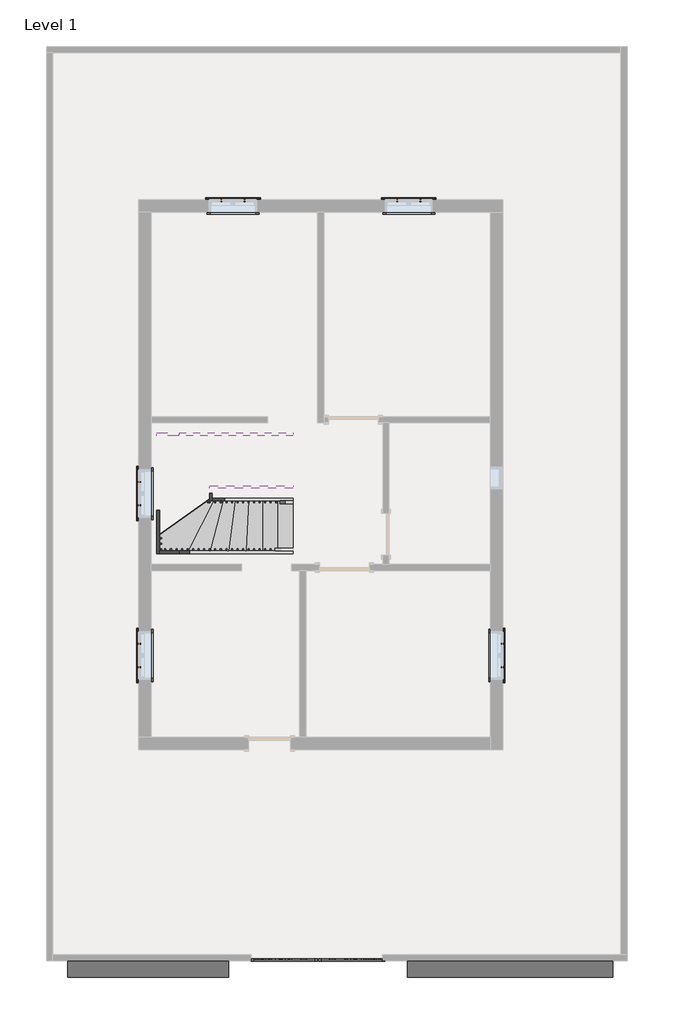
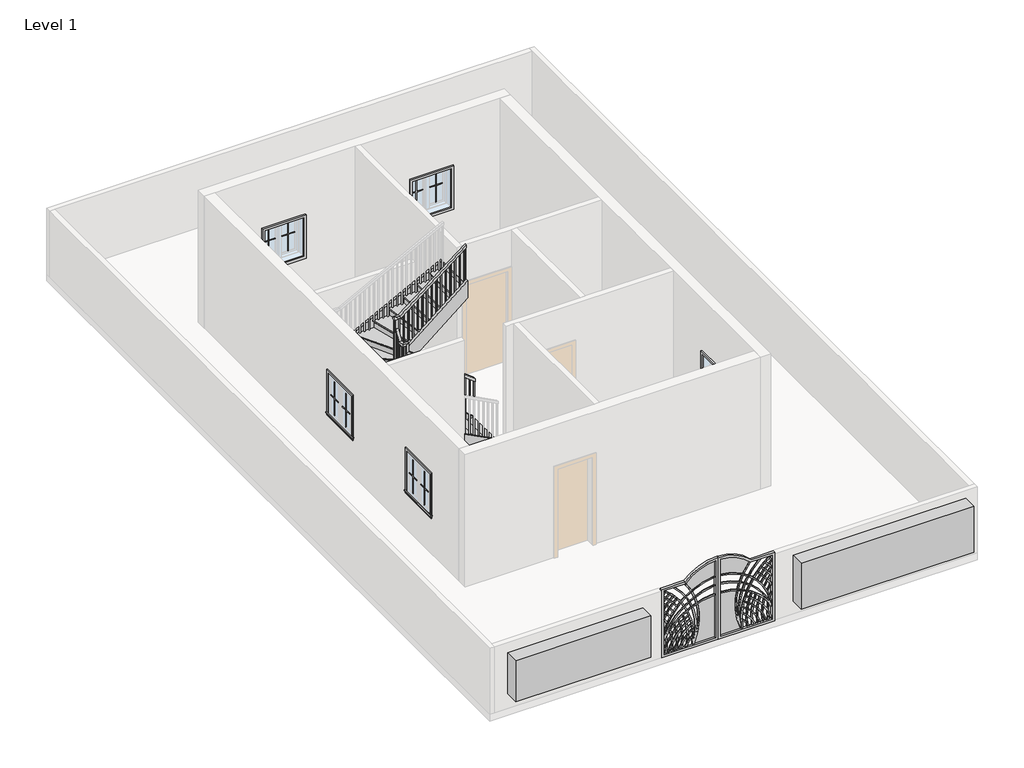
# One storey, part 2 of 2: 22 proxies, 8 members, 1 railing, 1 stair flight.
"""IFC4 building model written with IfcOpenShell, lengths in millimetres."""

from ifc_helpers import new_model, si_unit, frame, origin, place, context, project, spatial, polyline, outline, extrude, faceted_brep, transform, mapped, element, save
from components import generic_models_6bc30956, generic_models_1_generic_models_1_64d4bc32, muntin_pattern_2x2_muntin_pattern_2x2_b3fe6957, muntin_pattern_2x2_muntin_pattern_2x2_3e0ecaf2, trim_window_exterior_flat_with_sill_41619996, trim_window_interior_flat_picture_frame_51c85655, stair_flight_6f16d7d9

model = new_model("IFC4")

# Units and contexts
model_context = context("Model", 3, world=origin())
ifc_project = project(units=[si_unit("LENGTHUNIT", "METRE", prefix="MILLI")], contexts=[model_context])

# Site, building, storey
site = spatial("IfcSite", under=ifc_project)
building = spatial("IfcBuilding", under=site)
storey = spatial("IfcBuildingStorey", under=building, Name="Level 1", Elevation=0.0)

# Proxies
placement = place(None, origin())
generic_models_shape = generic_models_6bc30956(model_context)
element("IfcBuildingElementProxy", 1, Name="Generic Models", at=placement, inside=storey, context=model_context, shape_type="MappedRepresentation", body=[
    mapped(generic_models_shape, transform((-1329.9449167, -8721.9675636, 0.0), x_axis=(1.0, 0.0, 0.0), y_axis=(0.0, 1.0, 0.0), z_axis=(0.0, 0.0, 1.0))),
])
generic_models_1_generic_models_1_shape = generic_models_1_generic_models_1_64d4bc32(model_context)
element("IfcBuildingElementProxy", 2, Name="Generic Models 1 : Generic Models 1", ObjectType="Generic Models 1 : Generic Models 1", at=placement, inside=storey, context=model_context, shape_type="MappedRepresentation", body=[
    mapped(generic_models_1_generic_models_1_shape, transform((0.0, 0.0, 0.0), x_axis=(1.0, 0.0, 0.0), y_axis=(0.0, 1.0, 0.0), z_axis=(0.0, 0.0, 1.0))),
])
muntin_pattern_2x2_muntin_pattern_2x2_shape = muntin_pattern_2x2_muntin_pattern_2x2_b3fe6957(model_context)
element("IfcBuildingElementProxy", 3, Name="Muntin Pattern_2x2 : Muntin Pattern_2x2", ObjectType="Muntin Pattern_2x2 : Muntin Pattern_2x2", at=placement, inside=storey, context=model_context, shape_type="MappedRepresentation", body=[
    mapped(muntin_pattern_2x2_muntin_pattern_2x2_shape, transform((-3096.8324167, 5150.2179147, 984.25), x_axis=(1.0, 0.0, 0.0), y_axis=(0.0, 1.0, 0.0), z_axis=(0.0, 0.0, 1.0))),
])
element("IfcBuildingElementProxy", 4, Name="Muntin Pattern_2x2 : Muntin Pattern_2x2", ObjectType="Muntin Pattern_2x2 : Muntin Pattern_2x2", at=placement, inside=storey, context=model_context, shape_type="MappedRepresentation", body=[
    mapped(muntin_pattern_2x2_muntin_pattern_2x2_shape, transform((122.6175833, 5150.2179147, 984.25), x_axis=(1.0, 0.0, 0.0), y_axis=(0.0, 1.0, 0.0), z_axis=(0.0, 0.0, 1.0))),
])
element("IfcBuildingElementProxy", 5, Name="Muntin Pattern_2x2 : Muntin Pattern_2x2", ObjectType="Muntin Pattern_2x2 : Muntin Pattern_2x2", at=placement, inside=storey, context=model_context, shape_type="MappedRepresentation", body=[
    mapped(muntin_pattern_2x2_muntin_pattern_2x2_shape, transform((2051.4300833, -2960.3195853, 984.25), x_axis=(0.0, -1.0, 0.0), y_axis=(1.0, 0.0, 0.0), z_axis=(0.0, 0.0, 1.0))),
])
element("IfcBuildingElementProxy", 6, Name="Muntin Pattern_2x2 : Muntin Pattern_2x2", ObjectType="Muntin Pattern_2x2 : Muntin Pattern_2x2", at=placement, inside=storey, context=model_context, shape_type="MappedRepresentation", body=[
    mapped(muntin_pattern_2x2_muntin_pattern_2x2_shape, transform((-4597.0199167, -3388.9445853, 984.25), x_axis=(0.0, 1.0, 0.0), y_axis=(-1.0, 0.0, 0.0), z_axis=(0.0, 0.0, 1.0))),
])
element("IfcBuildingElementProxy", 7, Name="Muntin Pattern_2x2 : Muntin Pattern_2x2", ObjectType="Muntin Pattern_2x2 : Muntin Pattern_2x2", at=placement, inside=storey, context=model_context, shape_type="MappedRepresentation", body=[
    mapped(muntin_pattern_2x2_muntin_pattern_2x2_shape, transform((-4597.0199167, -426.6695853, 984.25), x_axis=(0.0, 1.0, 0.0), y_axis=(-1.0, 0.0, 0.0), z_axis=(0.0, 0.0, 1.0))),
])
muntin_pattern_2x2_muntin_pattern_2x2_2_shape = muntin_pattern_2x2_muntin_pattern_2x2_3e0ecaf2(model_context)
element("IfcBuildingElementProxy", 8, Name="Muntin Pattern_2x2 : Muntin Pattern_2x2", ObjectType="Muntin Pattern_2x2 : Muntin Pattern_2x2", at=placement, inside=storey, context=model_context, shape_type="MappedRepresentation", body=[
    mapped(muntin_pattern_2x2_muntin_pattern_2x2_2_shape, transform((-2668.2074167, 5150.2179147, 984.25), x_axis=(-1.0, 0.0, 0.0), y_axis=(0.0, -1.0, 0.0), z_axis=(0.0, 0.0, 1.0))),
])
element("IfcBuildingElementProxy", 9, Name="Muntin Pattern_2x2 : Muntin Pattern_2x2", ObjectType="Muntin Pattern_2x2 : Muntin Pattern_2x2", at=placement, inside=storey, context=model_context, shape_type="MappedRepresentation", body=[
    mapped(muntin_pattern_2x2_muntin_pattern_2x2_2_shape, transform((551.2425833, 5150.2179147, 984.25), x_axis=(-1.0, 0.0, 0.0), y_axis=(0.0, -1.0, 0.0), z_axis=(0.0, 0.0, 1.0))),
])
element("IfcBuildingElementProxy", 10, Name="Muntin Pattern_2x2 : Muntin Pattern_2x2", ObjectType="Muntin Pattern_2x2 : Muntin Pattern_2x2", at=placement, inside=storey, context=model_context, shape_type="MappedRepresentation", body=[
    mapped(muntin_pattern_2x2_muntin_pattern_2x2_2_shape, transform((2051.4300833, -3388.9445853, 984.25), x_axis=(0.0, 1.0, 0.0), y_axis=(-1.0, 0.0, 0.0), z_axis=(0.0, 0.0, 1.0))),
])
element("IfcBuildingElementProxy", 11, Name="Muntin Pattern_2x2 : Muntin Pattern_2x2", ObjectType="Muntin Pattern_2x2 : Muntin Pattern_2x2", at=placement, inside=storey, context=model_context, shape_type="MappedRepresentation", body=[
    mapped(muntin_pattern_2x2_muntin_pattern_2x2_2_shape, transform((-4597.0199167, -2960.3195853, 984.25), x_axis=(0.0, -1.0, 0.0), y_axis=(1.0, 0.0, 0.0), z_axis=(0.0, 0.0, 1.0))),
])
element("IfcBuildingElementProxy", 12, Name="Muntin Pattern_2x2 : Muntin Pattern_2x2", ObjectType="Muntin Pattern_2x2 : Muntin Pattern_2x2", at=placement, inside=storey, context=model_context, shape_type="MappedRepresentation", body=[
    mapped(muntin_pattern_2x2_muntin_pattern_2x2_2_shape, transform((-4597.0199167, 1.9554147, 984.25), x_axis=(0.0, -1.0, 0.0), y_axis=(1.0, 0.0, 0.0), z_axis=(0.0, 0.0, 1.0))),
])
trim_window_exterior_flat_with_sill_shape = trim_window_exterior_flat_with_sill_41619996(model_context)
element("IfcBuildingElementProxy", 13, Name="Trim-Window-Exterior-Flat : with Sill", ObjectType="Trim-Window-Exterior-Flat : with Sill", at=placement, inside=storey, context=model_context, shape_type="MappedRepresentation", body=[
    mapped(trim_window_exterior_flat_with_sill_shape, transform((-2882.5199167, 5159.7429147, 1828.8), x_axis=(-1.0, 0.0, 0.0), y_axis=(0.0, 0.0, 1.0), z_axis=(0.0, 1.0, 0.0))),
])
element("IfcBuildingElementProxy", 14, Name="Trim-Window-Exterior-Flat : with Sill", ObjectType="Trim-Window-Exterior-Flat : with Sill", at=placement, inside=storey, context=model_context, shape_type="MappedRepresentation", body=[
    mapped(trim_window_exterior_flat_with_sill_shape, transform((336.9300833, 5159.7429147, 1828.8), x_axis=(-1.0, 0.0, 0.0), y_axis=(0.0, 0.0, 1.0), z_axis=(0.0, 1.0, 0.0))),
])
element("IfcBuildingElementProxy", 15, Name="Trim-Window-Exterior-Flat : with Sill", ObjectType="Trim-Window-Exterior-Flat : with Sill", at=placement, inside=storey, context=model_context, shape_type="MappedRepresentation", body=[
    mapped(trim_window_exterior_flat_with_sill_shape, transform((2060.9550833, -3174.6320853, 1828.8), x_axis=(0.0, 1.0, 0.0), y_axis=(0.0, 0.0, 1.0), z_axis=(1.0, 0.0, 0.0))),
])
element("IfcBuildingElementProxy", 16, Name="Trim-Window-Exterior-Flat : with Sill", ObjectType="Trim-Window-Exterior-Flat : with Sill", at=placement, inside=storey, context=model_context, shape_type="MappedRepresentation", body=[
    mapped(trim_window_exterior_flat_with_sill_shape, transform((-4606.5449167, -3174.6320853, 1828.8), x_axis=(0.0, -1.0, 0.0), y_axis=(0.0, 0.0, 1.0), z_axis=(-1.0, 0.0, 0.0))),
])
element("IfcBuildingElementProxy", 17, Name="Trim-Window-Exterior-Flat : with Sill", ObjectType="Trim-Window-Exterior-Flat : with Sill", at=placement, inside=storey, context=model_context, shape_type="MappedRepresentation", body=[
    mapped(trim_window_exterior_flat_with_sill_shape, transform((-4606.5449167, -212.3570853, 1828.8), x_axis=(0.0, -1.0, 0.0), y_axis=(0.0, 0.0, 1.0), z_axis=(-1.0, 0.0, 0.0))),
])
trim_window_interior_flat_picture_frame_shape = trim_window_interior_flat_picture_frame_51c85655(model_context)
element("IfcBuildingElementProxy", 18, Name="Trim-Window-Interior-Flat : Picture Frame", ObjectType="Trim-Window-Interior-Flat : Picture Frame", at=placement, inside=storey, context=model_context, shape_type="MappedRepresentation", body=[
    mapped(trim_window_interior_flat_picture_frame_shape, transform((-2882.5199167, 4931.1429147, 1828.8), x_axis=(1.0, 0.0, 0.0), y_axis=(0.0, 0.0, 1.0), z_axis=(0.0, -1.0, 0.0))),
])
element("IfcBuildingElementProxy", 19, Name="Trim-Window-Interior-Flat : Picture Frame", ObjectType="Trim-Window-Interior-Flat : Picture Frame", at=placement, inside=storey, context=model_context, shape_type="MappedRepresentation", body=[
    mapped(trim_window_interior_flat_picture_frame_shape, transform((336.9300833, 4931.1429147, 1828.8), x_axis=(1.0, 0.0, 0.0), y_axis=(0.0, 0.0, 1.0), z_axis=(0.0, -1.0, 0.0))),
])
element("IfcBuildingElementProxy", 20, Name="Trim-Window-Interior-Flat : Picture Frame", ObjectType="Trim-Window-Interior-Flat : Picture Frame", at=placement, inside=storey, context=model_context, shape_type="MappedRepresentation", body=[
    mapped(trim_window_interior_flat_picture_frame_shape, transform((1832.3550833, -3174.6320853, 1828.8), x_axis=(0.0, -1.0, 0.0), y_axis=(0.0, 0.0, 1.0), z_axis=(-1.0, 0.0, 0.0))),
])
element("IfcBuildingElementProxy", 21, Name="Trim-Window-Interior-Flat : Picture Frame", ObjectType="Trim-Window-Interior-Flat : Picture Frame", at=placement, inside=storey, context=model_context, shape_type="MappedRepresentation", body=[
    mapped(trim_window_interior_flat_picture_frame_shape, transform((-4377.9449167, -3174.6320853, 1828.8), x_axis=(0.0, 1.0, 0.0), y_axis=(0.0, 0.0, 1.0), z_axis=(1.0, 0.0, 0.0))),
])
element("IfcBuildingElementProxy", 22, Name="Trim-Window-Interior-Flat : Picture Frame", ObjectType="Trim-Window-Interior-Flat : Picture Frame", at=placement, inside=storey, context=model_context, shape_type="MappedRepresentation", body=[
    mapped(trim_window_interior_flat_picture_frame_shape, transform((-4377.9449167, -212.3570853, 1828.8), x_axis=(0.0, 1.0, 0.0), y_axis=(0.0, 0.0, 1.0), z_axis=(1.0, 0.0, 0.0))),
])

# Members
element("IfcMember", 23, ObjectType="Stringer - 2\" Width", at=placement, inside=storey, context=model_context, shape_type="SweptSolid", body=[
    extrude(outline(polyline([(0.0, -1783.4132248), (229.639954, -1783.4132248), (1305.3956453, -3870.8304165), (962.500629, -3870.8304165), (0.0, -2003.1755424), (0.0, -1783.4132248)])), frame((0.0, -1310.9070853, 0.0), z_axis=(0.0, 1.0, 0.0), x_axis=(0.0, 0.0, 1.0)), (0.0, 0.0, 1.0), 50.8),
])
element("IfcMember", 24, ObjectType="Stringer - 2\" Width", at=placement, inside=storey, context=model_context, shape_type="SweptSolid", body=[
    extrude(outline(polyline([(-3870.8304165, -1260.1070853), (-3870.8304165, -1310.9070853), (-4225.5449167, -1310.9070853), (-4225.5449167, -1260.1070853), (-3870.8304165, -1260.1070853)])), frame((0.0, 0.0, 962.500629), z_axis=(0.0, 0.0, 1.0), x_axis=(1.0, 0.0, 0.0)), (0.0, 0.0, 1.0), 342.8950162),
])
element("IfcMember", 25, ObjectType="Stringer - 2\" Width", at=placement, inside=storey, context=model_context, shape_type="SweptSolid", body=[
    extrude(outline(polyline([(-1310.9070853, 1000.5956453), (-1310.9070853, 1289.0952212), (811.1127974, 1969.9972697), (848.0929147, 1969.9972697), (848.0929147, 1638.9682298), (-1141.3846024, 1000.5956453), (-1310.9070853, 1000.5956453)])), frame((-4276.3449167, 0.0, 0.0), z_axis=(1.0, 0.0, 0.0), x_axis=(0.0, 1.0, 0.0)), (0.0, 0.0, 1.0), 50.8),
])
element("IfcMember", 26, ObjectType="Stringer - 2\" Width", at=placement, inside=storey, context=model_context, shape_type="SweptSolid", body=[
    extrude(outline(polyline([(-4276.3449167, 848.0929147), (-4276.3449167, 898.8929147), (-3870.8304165, 898.8929147), (-3870.8304165, 848.0929147), (-4276.3449167, 848.0929147)])), frame((0.0, 0.0, 1649.8904473), z_axis=(0.0, 0.0, 1.0), x_axis=(1.0, 0.0, 0.0)), (0.0, 0.0, 1.0), 320.1068224),
])
element("IfcMember", 27, ObjectType="Stringer - 2\" Width", at=placement, inside=storey, context=model_context, shape_type="SweptSolid", body=[
    extrude(outline(polyline([(1969.9972697, -3870.8304165), (1649.8904473, -3870.8304165), (2725.6461385, -1783.4132248), (3045.7529609, -1783.4132248), (1969.9972697, -3870.8304165)])), frame((0.0, 848.0929147, 0.0), z_axis=(0.0, 1.0, 0.0), x_axis=(0.0, 0.0, 1.0)), (0.0, 0.0, 1.0), 50.8),
])
element("IfcMember", 28, ObjectType="Stringer - 2\" Width", at=placement, inside=storey, context=model_context, shape_type="SweptSolid", body=[
    extrude(outline(polyline([(0.0, -1783.4132248), (176.1764461, -1783.4132248), (1380.418648, -3260.3449167), (987.1410923, -3260.3449167), (0.0, -2049.6748694), (0.0, -1783.4132248)])), frame((0.0, -345.7070853, 0.0), z_axis=(0.0, 1.0, 0.0), x_axis=(0.0, 0.0, 1.0)), (0.0, 0.0, 1.0), 50.8),
])
element("IfcMember", 29, ObjectType="Stringer - 2\" Width", at=placement, inside=storey, context=model_context, shape_type="SweptSolid", body=[
    extrude(outline(polyline([(-345.7070853, 1028.5617647), (-345.7070853, 1573.2682978), (-139.0699679, 1926.1409689), (-117.1070853, 1926.1409689), (-117.1070853, 1360.465107), (-311.464868, 1028.5617647), (-345.7070853, 1028.5617647)])), frame((-3311.1449167, 0.0, 0.0), z_axis=(1.0, 0.0, 0.0), x_axis=(0.0, 1.0, 0.0)), (0.0, 0.0, 1.0), 50.8),
])
element("IfcMember", 30, ObjectType="Stringer - 2\" Width", at=placement, inside=storey, context=model_context, shape_type="SweptSolid", body=[
    extrude(outline(polyline([(1926.1409689, -3311.1449167), (1532.8634131, -3311.1449167), (2778.5262875, -1783.4132248), (3171.8038432, -1783.4132248), (1926.1409689, -3311.1449167)])), frame((0.0, -117.1070853, 0.0), z_axis=(0.0, 1.0, 0.0), x_axis=(0.0, 0.0, 1.0)), (0.0, 0.0, 1.0), 50.8),
])

# Railing
element("IfcRailing", 31, ObjectType="Handrail - Rectangular", at=placement, inside=storey, context=model_context, shape_type="SolidModel", body=[
    faceted_brep([(-1783.4132248, -396.5070853, 1083.7333333), (-1783.4132248, -396.5070853, 1019.4000346), (-1783.4132248, -345.7070853, 1019.4000346), (-1783.4132248, -345.7070853, 1083.7333333), (-3234.9449167, -396.5070853, 2211.6191036), (-3285.7449167, -396.5070853, 2186.7590024), (-3285.7449167, -345.7070853, 2186.7590024), (-3234.9449167, -345.7070853, 2211.6191036), (-3234.9449167, -396.5070853, 2414.6281882), (-3285.7449167, -396.5070853, 2363.8281882), (-3285.7449167, -345.7070853, 2363.8281882), (-3234.9449167, -345.7070853, 2414.6281882), (-3361.9449167, -396.5070853, 2414.6281882), (-3361.9449167, -396.5070853, 2363.8281882), (-3311.1449167, -345.7070853, 2363.8281882), (-3311.1449167, -345.7070853, 2414.6281882), (-3361.9449167, -269.5070853, 2414.6281882), (-3361.9449167, -240.3857515, 2363.8281882), (-3311.1449167, -240.3857515, 2363.8281882), (-3311.1449167, -269.5070853, 2414.6281882), (-3361.9449167, -142.5070853, 2631.5051451), (-3361.9449167, -91.7070853, 2617.7256424), (-3311.1449167, -91.7070853, 2617.7256424), (-3311.1449167, -142.5070853, 2631.5051451), (-3361.9449167, -142.5070853, 2834.5142297), (-3361.9449167, -91.7070853, 2783.7142297), (-3311.1449167, -91.7070853, 2783.7142297), (-3311.1449167, -142.5070853, 2834.5142297), (-3361.9449167, -15.5070853, 2834.5142297), (-3361.9449167, -15.5070853, 2783.7142297), (-3311.1449167, -66.3070853, 2783.7142297), (-3311.1449167, -66.3070853, 2834.5142297), (-3234.9449167, -15.5070853, 2834.5142297), (-3217.5282487, -15.5070853, 2783.7142297), (-3217.5282487, -66.3070853, 2783.7142297), (-3234.9449167, -66.3070853, 2834.5142297), (-1783.4132248, -15.5070853, 3962.4), (-1783.4132248, -66.3070853, 3962.4), (-1783.4132248, -66.3070853, 3898.0667013), (-1783.4132248, -15.5070853, 3898.0667013)], [[[0, 1, 2, 3]], [[1, 0, 4, 5]], [[2, 1, 5, 6]], [[3, 2, 6, 7]], [[0, 3, 7, 4]], [[5, 4, 8, 9]], [[6, 5, 9, 10]], [[7, 6, 10, 11]], [[4, 7, 11, 8]], [[9, 8, 12, 13]], [[10, 9, 13, 14]], [[11, 10, 14, 15]], [[8, 11, 15, 12]], [[13, 12, 16, 17]], [[14, 13, 17, 18]], [[15, 14, 18, 19]], [[12, 15, 19, 16]], [[17, 16, 20, 21]], [[18, 17, 21, 22]], [[19, 18, 22, 23]], [[16, 19, 23, 20]], [[21, 20, 24, 25]], [[22, 21, 25, 26]], [[23, 22, 26, 27]], [[20, 23, 27, 24]], [[25, 24, 28, 29]], [[26, 25, 29, 30]], [[27, 26, 30, 31]], [[24, 27, 31, 28]], [[29, 28, 32, 33]], [[30, 29, 33, 34]], [[31, 30, 34, 35]], [[28, 31, 35, 32]], [[36, 37, 38, 39]], [[33, 32, 36, 39]], [[34, 33, 39, 38]], [[35, 34, 38, 37]], [[32, 35, 37, 36]]]),
    extrude(outline(polyline([(3882.8316852, -1803.0199167), (3868.0292361, -1822.0699167), (2878.6666667, -1822.0699167), (2878.6666667, -1803.0199167), (3882.8316852, -1803.0199167)])), frame((0.0, -50.4320853, 0.0), z_axis=(0.0, 1.0, 0.0), x_axis=(0.0, 0.0, 1.0)), (0.0, 0.0, 1.0), 19.05),
    extrude(outline(polyline([(3803.8852902, -1904.6199167), (3789.0828411, -1923.6699167), (2878.6666667, -1923.6699167), (2878.6666667, -1904.6199167), (3803.8852902, -1904.6199167)])), frame((0.0, -50.4320853, 0.0), z_axis=(0.0, 1.0, 0.0), x_axis=(0.0, 0.0, 1.0)), (0.0, 0.0, 1.0), 19.05),
    extrude(outline(polyline([(3724.9388952, -2006.2199167), (3710.1364462, -2025.2699167), (2878.6666667, -2025.2699167), (2878.6666667, -2006.2199167), (3724.9388952, -2006.2199167)])), frame((0.0, -50.4320853, 0.0), z_axis=(0.0, 1.0, 0.0), x_axis=(0.0, 0.0, 1.0)), (0.0, 0.0, 1.0), 19.05),
    extrude(outline(polyline([(3645.9925003, -2107.8199167), (3631.1900512, -2126.8699167), (2709.3333333, -2126.8699167), (2709.3333333, -2107.8199167), (3645.9925003, -2107.8199167)])), frame((0.0, -50.4320853, 0.0), z_axis=(0.0, 1.0, 0.0), x_axis=(0.0, 0.0, 1.0)), (0.0, 0.0, 1.0), 19.05),
    extrude(outline(polyline([(3567.0461053, -2209.4199167), (3552.2436562, -2228.4699167), (2709.3333333, -2228.4699167), (2709.3333333, -2209.4199167), (3567.0461053, -2209.4199167)])), frame((0.0, -50.4320853, 0.0), z_axis=(0.0, 1.0, 0.0), x_axis=(0.0, 0.0, 1.0)), (0.0, 0.0, 1.0), 19.05),
    extrude(outline(polyline([(3488.0997103, -2311.0199167), (3473.2972613, -2330.0699167), (2709.3333333, -2330.0699167), (2709.3333333, -2311.0199167), (3488.0997103, -2311.0199167)])), frame((0.0, -50.4320853, 0.0), z_axis=(0.0, 1.0, 0.0), x_axis=(0.0, 0.0, 1.0)), (0.0, 0.0, 1.0), 19.05),
    extrude(outline(polyline([(3409.1533154, -2412.6199167), (3394.3508663, -2431.6699167), (2540.0, -2431.6699167), (2540.0, -2412.6199167), (3409.1533154, -2412.6199167)])), frame((0.0, -50.4320853, 0.0), z_axis=(0.0, 1.0, 0.0), x_axis=(0.0, 0.0, 1.0)), (0.0, 0.0, 1.0), 19.05),
    extrude(outline(polyline([(3330.2069204, -2514.2199167), (3315.4044713, -2533.2699167), (2540.0, -2533.2699167), (2540.0, -2514.2199167), (3330.2069204, -2514.2199167)])), frame((0.0, -50.4320853, 0.0), z_axis=(0.0, 1.0, 0.0), x_axis=(0.0, 0.0, 1.0)), (0.0, 0.0, 1.0), 19.05),
    extrude(outline(polyline([(3251.2605254, -2615.8199167), (3236.4580764, -2634.8699167), (2370.6666667, -2634.8699167), (2370.6666667, -2615.8199167), (3251.2605254, -2615.8199167)])), frame((0.0, -50.4320853, 0.0), z_axis=(0.0, 1.0, 0.0), x_axis=(0.0, 0.0, 1.0)), (0.0, 0.0, 1.0), 19.05),
    extrude(outline(polyline([(3172.3141304, -2717.4199167), (3157.5116814, -2736.4699167), (2370.6666667, -2736.4699167), (2370.6666667, -2717.4199167), (3172.3141304, -2717.4199167)])), frame((0.0, -50.4320853, 0.0), z_axis=(0.0, 1.0, 0.0), x_axis=(0.0, 0.0, 1.0)), (0.0, 0.0, 1.0), 19.05),
    extrude(outline(polyline([(3093.3677355, -2819.0199167), (3078.5652864, -2838.0699167), (2370.6666667, -2838.0699167), (2370.6666667, -2819.0199167), (3093.3677355, -2819.0199167)])), frame((0.0, -50.4320853, 0.0), z_axis=(0.0, 1.0, 0.0), x_axis=(0.0, 0.0, 1.0)), (0.0, 0.0, 1.0), 19.05),
    extrude(outline(polyline([(3014.4213405, -2920.6199167), (2999.6188914, -2939.6699167), (2201.3333333, -2939.6699167), (2201.3333333, -2920.6199167), (3014.4213405, -2920.6199167)])), frame((0.0, -50.4320853, 0.0), z_axis=(0.0, 1.0, 0.0), x_axis=(0.0, 0.0, 1.0)), (0.0, 0.0, 1.0), 19.05),
    extrude(outline(polyline([(2935.4749455, -3022.2199167), (2920.6724965, -3041.2699167), (2201.3333333, -3041.2699167), (2201.3333333, -3022.2199167), (2935.4749455, -3022.2199167)])), frame((0.0, -50.4320853, 0.0), z_axis=(0.0, 1.0, 0.0), x_axis=(0.0, 0.0, 1.0)), (0.0, 0.0, 1.0), 19.05),
    extrude(outline(polyline([(2856.5285506, -3123.8199167), (2841.7261015, -3142.8699167), (2032.0, -3142.8699167), (2032.0, -3123.8199167), (2856.5285506, -3123.8199167)])), frame((0.0, -50.4320853, 0.0), z_axis=(0.0, 1.0, 0.0), x_axis=(0.0, 0.0, 1.0)), (0.0, 0.0, 1.0), 19.05),
    extrude(outline(polyline([(2777.5821556, -3225.4199167), (2762.7797065, -3244.4699167), (2032.0, -3244.4699167), (2032.0, -3225.4199167), (2777.5821556, -3225.4199167)])), frame((0.0, -50.4320853, 0.0), z_axis=(0.0, 1.0, 0.0), x_axis=(0.0, 0.0, 1.0)), (0.0, 0.0, 1.0), 19.05),
    extrude(outline(polyline([(-3327.0199167, -75.8320853), (-3346.0699167, -75.8320853), (-3346.0699167, -56.7820853), (-3327.0199167, -56.7820853), (-3327.0199167, -75.8320853)])), frame((0.0, 0.0, 1693.3333333), z_axis=(0.0, 0.0, 1.0), x_axis=(1.0, 0.0, 0.0)), (0.0, 0.0, 1.0), 1090.3808964),
    extrude(outline(polyline([(-177.4320853, 2471.3336964), (-158.3820853, 2503.86524), (-158.3820853, 1524.0), (-177.4320853, 1524.0), (-177.4320853, 2471.3336964)])), frame((-3346.0699167, 0.0, 0.0), z_axis=(1.0, 0.0, 0.0), x_axis=(0.0, 1.0, 0.0)), (0.0, 0.0, 1.0), 19.05),
    extrude(outline(polyline([(-279.0320853, 2297.8321309), (-259.9820853, 2330.3636744), (-259.9820853, 1354.6666667), (-279.0320853, 1354.6666667), (-279.0320853, 2297.8321309)])), frame((-3346.0699167, 0.0, 0.0), z_axis=(1.0, 0.0, 0.0), x_axis=(0.0, 1.0, 0.0)), (0.0, 0.0, 1.0), 19.05),
    extrude(outline(polyline([(-3297.8882248, -361.5820853), (-3297.8882248, -380.6320853), (-3316.9382248, -380.6320853), (-3316.9382248, -361.5820853), (-3297.8882248, -361.5820853)])), frame((0.0, 0.0, 1185.3333333), z_axis=(0.0, 0.0, 1.0), x_axis=(1.0, 0.0, 0.0)), (0.0, 0.0, 1.0), 1178.4948549),
    extrude(outline(polyline([(2117.2483397, -3196.2882248), (2132.0507888, -3215.3382248), (1016.0, -3215.3382248), (1016.0, -3196.2882248), (2117.2483397, -3196.2882248)])), frame((0.0, -380.6320853, 0.0), z_axis=(0.0, 1.0, 0.0), x_axis=(0.0, 0.0, 1.0)), (0.0, 0.0, 1.0), 19.05),
    extrude(outline(polyline([(2038.3019447, -3094.6882248), (2053.1043938, -3113.7382248), (1016.0, -3113.7382248), (1016.0, -3094.6882248), (2038.3019447, -3094.6882248)])), frame((0.0, -380.6320853, 0.0), z_axis=(0.0, 1.0, 0.0), x_axis=(0.0, 0.0, 1.0)), (0.0, 0.0, 1.0), 19.05),
    extrude(outline(polyline([(1959.3555498, -2993.0882248), (1974.1579988, -3012.1382248), (846.6666667, -3012.1382248), (846.6666667, -2993.0882248), (1959.3555498, -2993.0882248)])), frame((0.0, -380.6320853, 0.0), z_axis=(0.0, 1.0, 0.0), x_axis=(0.0, 0.0, 1.0)), (0.0, 0.0, 1.0), 19.05),
    extrude(outline(polyline([(1880.4091548, -2891.4882248), (1895.2116039, -2910.5382248), (846.6666667, -2910.5382248), (846.6666667, -2891.4882248), (1880.4091548, -2891.4882248)])), frame((0.0, -380.6320853, 0.0), z_axis=(0.0, 1.0, 0.0), x_axis=(0.0, 0.0, 1.0)), (0.0, 0.0, 1.0), 19.05),
    extrude(outline(polyline([(1801.4627598, -2789.8882248), (1816.2652089, -2808.9382248), (677.3333333, -2808.9382248), (677.3333333, -2789.8882248), (1801.4627598, -2789.8882248)])), frame((0.0, -380.6320853, 0.0), z_axis=(0.0, 1.0, 0.0), x_axis=(0.0, 0.0, 1.0)), (0.0, 0.0, 1.0), 19.05),
    extrude(outline(polyline([(1722.5163649, -2688.2882248), (1737.3188139, -2707.3382248), (677.3333333, -2707.3382248), (677.3333333, -2688.2882248), (1722.5163649, -2688.2882248)])), frame((0.0, -380.6320853, 0.0), z_axis=(0.0, 1.0, 0.0), x_axis=(0.0, 0.0, 1.0)), (0.0, 0.0, 1.0), 19.05),
    extrude(outline(polyline([(1643.5699699, -2586.6882248), (1658.3724189, -2605.7382248), (508.0, -2605.7382248), (508.0, -2586.6882248), (1643.5699699, -2586.6882248)])), frame((0.0, -380.6320853, 0.0), z_axis=(0.0, 1.0, 0.0), x_axis=(0.0, 0.0, 1.0)), (0.0, 0.0, 1.0), 19.05),
    extrude(outline(polyline([(1564.6235749, -2485.0882248), (1579.426024, -2504.1382248), (508.0, -2504.1382248), (508.0, -2485.0882248), (1564.6235749, -2485.0882248)])), frame((0.0, -380.6320853, 0.0), z_axis=(0.0, 1.0, 0.0), x_axis=(0.0, 0.0, 1.0)), (0.0, 0.0, 1.0), 19.05),
    extrude(outline(polyline([(1485.6771799, -2383.4882248), (1500.479629, -2402.5382248), (508.0, -2402.5382248), (508.0, -2383.4882248), (1485.6771799, -2383.4882248)])), frame((0.0, -380.6320853, 0.0), z_axis=(0.0, 1.0, 0.0), x_axis=(0.0, 0.0, 1.0)), (0.0, 0.0, 1.0), 19.05),
    extrude(outline(polyline([(1406.730785, -2281.8882248), (1421.533234, -2300.9382248), (338.6666667, -2300.9382248), (338.6666667, -2281.8882248), (1406.730785, -2281.8882248)])), frame((0.0, -380.6320853, 0.0), z_axis=(0.0, 1.0, 0.0), x_axis=(0.0, 0.0, 1.0)), (0.0, 0.0, 1.0), 19.05),
    extrude(outline(polyline([(1327.78439, -2180.2882248), (1342.5868391, -2199.3382248), (338.6666667, -2199.3382248), (338.6666667, -2180.2882248), (1327.78439, -2180.2882248)])), frame((0.0, -380.6320853, 0.0), z_axis=(0.0, 1.0, 0.0), x_axis=(0.0, 0.0, 1.0)), (0.0, 0.0, 1.0), 19.05),
    extrude(outline(polyline([(1248.837995, -2078.6882248), (1263.6404441, -2097.7382248), (338.6666667, -2097.7382248), (338.6666667, -2078.6882248), (1248.837995, -2078.6882248)])), frame((0.0, -380.6320853, 0.0), z_axis=(0.0, 1.0, 0.0), x_axis=(0.0, 0.0, 1.0)), (0.0, 0.0, 1.0), 19.05),
    extrude(outline(polyline([(1169.8916001, -1977.0882248), (1184.6940491, -1996.1382248), (169.3333333, -1996.1382248), (169.3333333, -1977.0882248), (1169.8916001, -1977.0882248)])), frame((0.0, -380.6320853, 0.0), z_axis=(0.0, 1.0, 0.0), x_axis=(0.0, 0.0, 1.0)), (0.0, 0.0, 1.0), 19.05),
    extrude(outline(polyline([(1090.9452051, -1875.4882248), (1105.7476541, -1894.5382248), (169.3333333, -1894.5382248), (169.3333333, -1875.4882248), (1090.9452051, -1875.4882248)])), frame((0.0, -380.6320853, 0.0), z_axis=(0.0, 1.0, 0.0), x_axis=(0.0, 0.0, 1.0)), (0.0, 0.0, 1.0), 19.05),
    extrude(outline(polyline([(-3327.0199167, -50.4320853), (-3346.0699167, -50.4320853), (-3346.0699167, -31.3820853), (-3327.0199167, -31.3820853), (-3327.0199167, -50.4320853)])), frame((0.0, 0.0, 1862.6666667), z_axis=(0.0, 0.0, 1.0), x_axis=(1.0, 0.0, 0.0)), (0.0, 0.0, 1.0), 921.0475631),
    extrude(outline(polyline([(-3327.0199167, -361.5820853), (-3327.0199167, -380.6320853), (-3346.0699167, -380.6320853), (-3346.0699167, -361.5820853), (-3327.0199167, -361.5820853)])), frame((0.0, 0.0, 1185.3333333), z_axis=(0.0, 0.0, 1.0), x_axis=(1.0, 0.0, 0.0)), (0.0, 0.0, 1.0), 1178.4948549),
    extrude(outline(polyline([(3898.0667013, -1783.4132248), (3883.2642523, -1802.4632248), (2878.6666667, -1802.4632248), (2878.6666667, -1783.4132248), (3898.0667013, -1783.4132248)])), frame((0.0, -50.4320853, 0.0), z_axis=(0.0, 1.0, 0.0), x_axis=(0.0, 0.0, 1.0)), (0.0, 0.0, 1.0), 19.05),
    extrude(outline(polyline([(1019.4000346, -1783.4132248), (1034.2024837, -1802.4632248), (169.3333333, -1802.4632248), (169.3333333, -1783.4132248), (1019.4000346, -1783.4132248)])), frame((0.0, -380.6320853, 0.0), z_axis=(0.0, 1.0, 0.0), x_axis=(0.0, 0.0, 1.0)), (0.0, 0.0, 1.0), 19.05),
])

# Stair flight
stair_flight_shape = stair_flight_6f16d7d9(model_context)
element("IfcStairFlight", 32, ObjectType="2\" Tread 1\" Nosing 1/4\" Riser", at=placement, inside=storey, context=model_context, shape_type="MappedRepresentation", body=[
    mapped(stair_flight_shape, transform((0.0, 0.0, 0.0), x_axis=(1.0, 0.0, 0.0), y_axis=(0.0, 1.0, 0.0), z_axis=(0.0, 0.0, 1.0))),
])

save(model, "model.ifc")

# Revit data of these elements
# Type
#   m.s. sheet = none
#   2" x2" pipe = none
#   1"x1"pipe = none
#   Default Elevation = 0
# Type "Muntin Pattern_2x2 : Muntin Pattern_2x2"
#   Width [instance default] = 4' - 0"
#   Thickness = 0' - 0 1/2"
#   Height [instance default] = 4' - 0"
#   Distance = 0' - 0 3/4"
#   Interior Material [instance default] = none
#   Exterior Material [instance default] = none
#   Default Elevation = 0
# Type "Trim-Window-Exterior-Flat : with Sill"
#   Trim Width = 0' - 2 1/4"
#   Trim Thickness_Picture Frame = 0' - 1 1/4"
#   Trim Thickness_with Sill = 0' - 0 3/4"
#   Sill Thickness = 0' - 1 1/4"
#   Opening Width [instance default] = 2' - 0"
#   Opening Height [instance default] = 3' - 0"
#   Default Elevation = 4' - 0"
#   Sill = yes
#   Picture Frame = no
#   Trim Material [instance default] = none
# Type "Trim-Window-Interior-Flat : Picture Frame"
#   Trim Thickness_Picture Frame = 0' - 1 1/4"
#   Trim Width = 0' - 2 1/4"
#   Trim Thickness_with Sill = 0' - 0 3/4"
#   Sill Thickness = 0' - 1 1/4"
#   Opening Width [instance default] = 2' - 0"
#   Opening Height [instance default] = 3' - 0"
#   Default Elevation = 4' - 0"
#   Sill = no
#   Picture Frame = yes
#   Trim Material [instance default] = none
# Type "Handrail - Rectangular"
#   Assembly Code = "C2010400"
#   built-in parameter 1008612 = 0.0416667 (stored number, unit not read)
#   built-in parameter 1008611 = 0.0416667 (stored number, unit not read)
#   built-in parameter 1008609 = 0.333333 (stored number, unit not read)
#   built-in parameter 1008604 = 0.166667 (stored number, unit not read)
#   built-in parameter 1008603 = 0.166667 (stored number, unit not read)
#   Railing Height = 3' - 0"
#   built-in parameter 1008630 = 2
#   built-in parameter 1008610 = 2
#   built-in parameter 1008618 = Baluster - Square : 3/4"
# Element 1 (IfcBuildingElementProxy)
#   Phase Created = New Construction
#   Materials on its faces: "r1"
# Element 2 (IfcBuildingElementProxy, "Generic Models 1 : Generic Models 1")
#   Phase Created = New Construction
#   Materials on its faces: "Parking Stripe"
# Elements 3, 4, 5, 6, 7, 8, 9, 10, 11, 12 (IfcBuildingElementProxy, "Muntin Pattern_2x2 : Muntin Pattern_2x2")
#   Width = 0' - 11 5/8"
#   Height = 2' - 6 1/2"
#   Interior Material = Wood - Stained
#   Exterior Material = Clad - White
#   Phase Created = New Construction
#   Materials on its faces: "Clad - White", "Wood - Stained"
# Elements 13, 14, 15, 16, 17 (IfcBuildingElementProxy, "Trim-Window-Exterior-Flat : with Sill")
#   Opening Width = 2' - 10"
#   Opening Height = 3' - 0"
#   Trim Material = Clad - White
#   Phase Created = New Construction
#   Materials on its faces: "Clad - White"
# Elements 18, 19, 20, 21, 22 (IfcBuildingElementProxy, "Trim-Window-Interior-Flat : Picture Frame")
#   Opening Width = 2' - 10"
#   Opening Height = 3' - 0"
#   Trim Material = Wood - Stained
#   Phase Created = New Construction
#   Materials on its faces: "Wood - Stained"
# Elements 23, 24, 25, 26, 27, 28, 29, 30 (IfcMember, "Stringer - 2\" Width")
#   Phase Created = New Construction
# Element 31 (IfcRailing, "Handrail - Rectangular")
#   Phase Created = New Construction
# Element 32 (IfcStairFlight, "2\" Tread 1\" Nosing 1/4\" Riser")
#   Phase Created = New Construction
# Materials
#   "r1": class "Generic", colour RGB 120 120 120, transparency 0, Cost = 0
#   "Parking Stripe": class "Paint", colour RGB 250 250 91, transparency 0, Cost = 0
#   "Clad - White": class "Wood", colour RGB 242 242 238, transparency 0, Cost = 0
#   "Wood - Stained": class "Wood", colour RGB 224 178 126, transparency 0, Cost = 0
